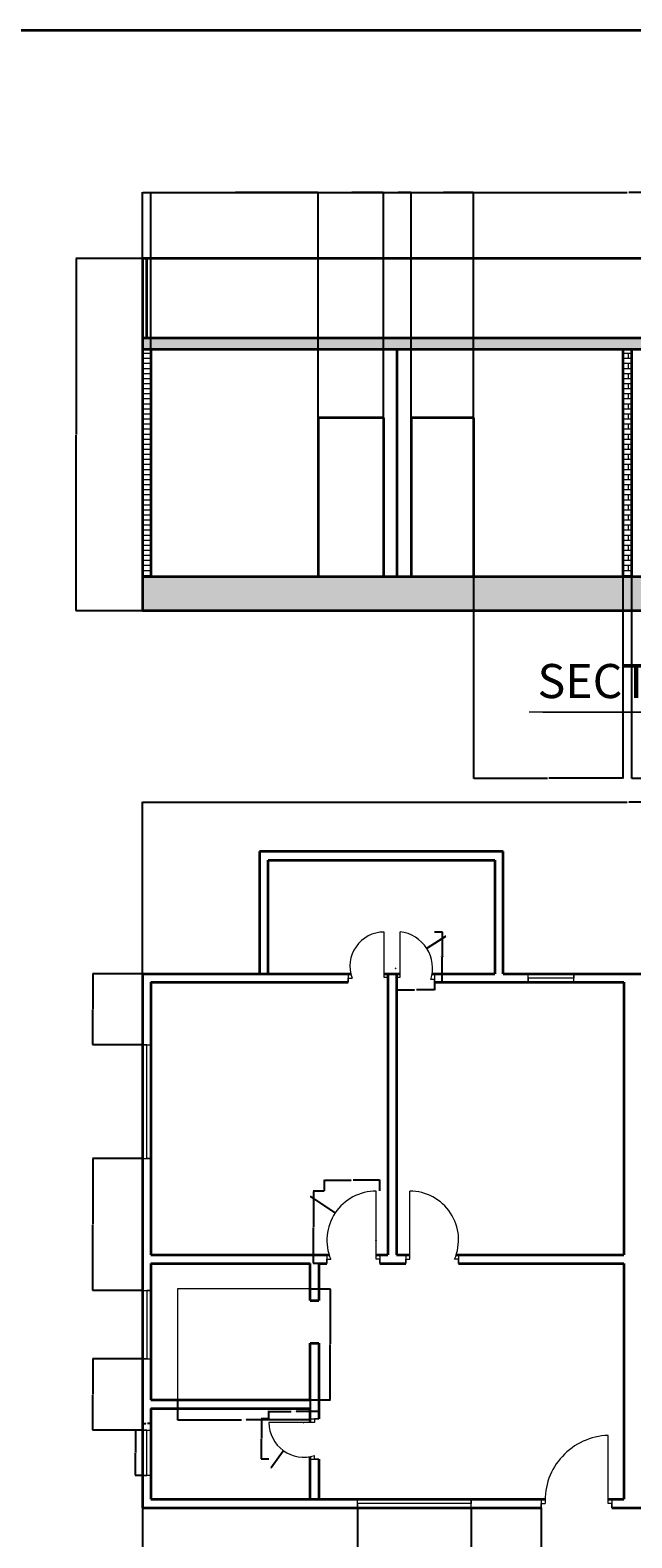
# Model space of a CAD drawing. Units: inches. Extents: x 2055 to 3558, y 1520 to 2888.
# Tile 7 of 8: x 2732 to 3050, y 2092 to 2888. Entities that reach past the tile are written whole.
import ezdxf

# ---------------------------------------------------------------- set-up
doc = ezdxf.new("R2010")
doc.units = ezdxf.units.IN
for name, color, linetype, lineweight in [('A-ANNO-DIMS', 2, 'Continuous', 18), ('A-ANNO-TEXT', 7, 'Continuous', 18), ('A-ANNO-TTLB', 7, 'Continuous', 35), ('A-DOOR', 3, 'Continuous', 18), ('A-FLOR-FIXT', 8, 'Continuous', 18), ('A-GLAZ', 4, 'Continuous', 18), ('A-SECT', 7, 'Continuous', 35), ('A-SECT-PATT', 252, 'Continuous', 13), ('A-WALL', 7, 'Continuous', 35), ('A-WALL-PATT', 252, 'Continuous', 13)]:
    doc.layers.add(name, color=color, linetype=linetype, lineweight=lineweight)
doc.styles.get("Standard").update_dxf_attribs({"font": 'arial.ttf'})
doc.dimstyles.get("Standard").update_dxf_attribs({"dimtxt": 0.18, "dimasz": 0.18, "dimexe": 0.18, "dimexo": 0.0625, "dimgap": 0.09, "dimtad": 0, "dimtih": 1, "dimtoh": 1, "dimdec": 4, "dimzin": 0, "dimdsep": 46, "dimtxsty": 'Standard', "dimcen": 0.09, "dimadec": 0, "dimazin": 0, "dimtfac": 1, "dimtdec": 4, "dimtofl": 0, "dimtmove": 0, "dimatfit": 3, "dimfxl": 1, "dimtolj": 1, "dimtzin": 0, "dimarcsym": 0})

# ---------------------------------------------------------------- blocks, each defined once
blk = doc.blocks.new('DOOR-BED-36-A')
for p, q in [((26, 2.25), (26, 38.25)), ((0, 4.5), (0, 0)), ((0, 0), (0, 2.25)), ((0, 2.25), (2, 2.25)), ((28, 2.25), (26, 2.25)), ((28, 4.5), (28, 0)), ((28, 0), (28, 2.25))]:
    blk.add_line(p, q)
blk.add_arc((26, 12.25), 26, 90, 202.62954)
blk = doc.blocks.new('DOOR-BED-36-B')
for p, q in [((2, 2.25), (2, 38.25)), ((0, 4.5), (0, 0)), ((0, 0), (0, 2.25)), ((0, 2.25), (2, 2.25)), ((27.66, 2.25), (25.66, 2.25)), ((27.66, 4.5), (27.66, 0)), ((27.66, 0), (27.66, 2.25))]:
    blk.add_line(p, q)
blk.add_arc((2, 12.47), 25.78, 336.6346, 90)
blk = doc.blocks.new('DOOR-ENTRY-36-B')
for p, q in [((35.2, 2.25), (35.2, 38.25)), ((0, 4.5), (0, 0)), ((0, 0), (0, 2.25)), ((0, 2.25), (2, 2.25)), ((37.2, 2.25), (35.2, 2.25)), ((37.2, 4.5), (37.2, 0)), ((37.2, 0), (37.2, 2.25))]:
    blk.add_line(p, q)
blk.add_arc((36.42, 3.82), 34.45, 92.03168, 182.60616)
blk = doc.blocks.new('DOOR-VERANDA-24-E')
for p, q in [((2, 2.71), (2, 26.71)), ((0, 2.71), (2, 2.71)), ((20.12, 1.44), (18.12, 1.44)), ((20.12, 4.5), (20.12, 0)), ((20.12, 0), (20.12, 1.44))]:
    blk.add_line(p, q)
blk.add_arc((-0.34, 7.44), 19.42, 342.01317, 83.06507)
blk = doc.blocks.new('DOOR-VERANDA-24-F')
for p, q in [((18.85, 2.51), (18.85, 26.51)), ((0, 4.5), (0, 0)), ((0, 0), (0, 2.25)), ((0, 2.25), (2, 2.25)), ((20.85, 2.51), (18.85, 2.51))]:
    blk.add_line(p, q)
blk.add_arc((18.85, 8.53), 17.98, 90, 200.4386)
blk = doc.blocks.new('DOOR-BATH-24-D')
for p, q in [((24, 19.33), (0, 19.33)), ((21.75, 21.33), (26.25, 21.33)), ((26.25, 21.33), (24, 21.33)), ((24, 21.33), (24, 19.33)), ((21.75, 0), (26.25, 0)), ((24, 0), (24, 2)), ((26.25, 0), (24, 0))]:
    blk.add_line(p, q)
blk.add_arc((18.26, 19.33), 18.26, 180, 288.33755)
blk = doc.blocks.new('WIN-36')
for p, q in [((2.25, 36), (0, 36)), ((0, 36), (4.5, 36)), ((2.25, 0), (2.25, 36)), ((0, 0), (4.5, 0)), ((4.5, 0), (2.25, 0))]:
    blk.add_line(p, q)
blk = doc.blocks.new('WIN-24')
for p, q in [((0, 24), (4.5, 24)), ((4.5, 24), (2.25, 24)), ((2.25, 24), (2.25, 0)), ((2.25, 0), (0, 0)), ((0, 0), (4.5, 0))]:
    blk.add_line(p, q)
blk = doc.blocks.new('WIN-24-2')
for p, q in [((2.25, 24), (0, 24)), ((0, 24), (4.5, 24)), ((2.25, 0), (2.25, 24)), ((4.5, 0), (0, 0)), ((0, 0), (2.25, 0))]:
    blk.add_line(p, q)
blk = doc.blocks.new('WIN-60')
for p, q in [((0, 60), (4.5, 60)), ((4.5, 60), (2.25, 60)), ((2.25, 60), (2.25, 0)), ((2.25, 0), (0, 0)), ((0, 0), (4.5, 0))]:
    blk.add_line(p, q)
blk = doc.blocks.new('COUNTER-1')
for p, q in [((70.02, 58.69), (0, 58.69)), ((0, 58.69), (0, 0))]:
    blk.add_line(p, q)
blk = doc.blocks.new('VERANDA-PERIMETER')
for p, q in [((0, 0), (0, 64.5)), ((4.5, 64.5), (4.5, 4.5)), ((124.15, 4.5), (124.15, 64.5)), ((128.65, 64.5), (128.65, 4.5)), ((4.5, 0), (0, 0)), ((4.5, 4.5), (124.15, 4.5)), ((128.65, 0), (4.5, 0)), ((128.65, 4.5), (128.65, 0))]:
    blk.add_line(p, q)
blk = doc.blocks.new('*D52')
at = {"layer": 'A-ANNO-DIMS', "color": 0, "lineweight": -2, "transparency": 16777216}
for p, q in [((2887.43, 2275.25), (2881.58, 2275.25)), ((2881.76, 2275.07), (2881.76, 2256.31)), ((2881.76, 2237.18), (2881.76, 2255.94)), ((2887.43, 2237), (2881.58, 2237))]:
    blk.add_line(p, q, dxfattribs=at)
at = {"layer": 'A-ANNO-DIMS', "color": 0, "transparency": 16777216}
for points in [[(2881.73, 2275.07), (2881.79, 2275.07), (2881.76, 2275.25)], [(2881.73, 2237.18), (2881.79, 2237.18), (2881.76, 2237)]]:
    blk.add_solid(points, dxfattribs=at)
at = {"layer": 'Defpoints', "color": 0, "transparency": 16777216}
for p in [(2881.76, 2275.25), (2887.49, 2275.25), (2887.49, 2237)]:
    blk.add_point(p, dxfattribs=at)
at = {"layer": 'A-ANNO-DIMS', "color": 0, "transparency": 16777216, "insert": (2881.76, 2256.12), "char_height": 0.18, "attachment_point": 5}
blk.add_mtext('\\A1;BED DOOR 38 TYP.', dxfattribs=at)
blk = doc.blocks.new('*D53')
at = {"layer": 'A-ANNO-DIMS', "color": 0, "lineweight": -2, "transparency": 16777216}
for p, q in [((2887.49, 2275.31), (2887.49, 2281.17)), ((2887.67, 2280.99), (2901.63, 2280.99)), ((2916.65, 2280.99), (2902.69, 2280.99)), ((2916.83, 2275.31), (2916.83, 2281.17))]:
    blk.add_line(p, q, dxfattribs=at)
at = {"layer": 'A-ANNO-DIMS', "color": 0, "transparency": 16777216}
for points in [[(2887.67, 2281.02), (2887.67, 2280.96), (2887.49, 2280.99)], [(2916.65, 2281.02), (2916.65, 2280.96), (2916.83, 2280.99)]]:
    blk.add_solid(points, dxfattribs=at)
at = {"layer": 'Defpoints', "color": 0, "transparency": 16777216}
for p in [(2916.83, 2280.99), (2887.49, 2275.25), (2916.83, 2275.25)]:
    blk.add_point(p, dxfattribs=at)
at = {"layer": 'A-ANNO-DIMS', "color": 0, "transparency": 16777216, "insert": (2902.16, 2280.99), "char_height": 0.18, "attachment_point": 5}
blk.add_mtext('\\A1;29 TYP.', dxfattribs=at)
blk = doc.blocks.new('*D90')
at = {"layer": 'A-ANNO-DIMS', "color": 0, "lineweight": -2, "transparency": 16777216}
for p, q in [((2945.68, 2412.21), (2949.81, 2412.21)), ((2949.63, 2412.03), (2949.63, 2399.04)), ((2949.63, 2385.68), (2949.63, 2398.67)), ((2945.68, 2385.5), (2949.81, 2385.5))]:
    blk.add_line(p, q, dxfattribs=at)
at = {"layer": 'A-ANNO-DIMS', "color": 0, "transparency": 16777216}
for points in [[(2949.6, 2412.03), (2949.66, 2412.03), (2949.63, 2412.21)], [(2949.6, 2385.68), (2949.66, 2385.68), (2949.63, 2385.5)]]:
    blk.add_solid(points, dxfattribs=at)
at = {"layer": 'Defpoints', "color": 0, "transparency": 16777216}
for p in [(2945.62, 2412.21), (2949.63, 2412.21), (2945.62, 2385.5)]:
    blk.add_point(p, dxfattribs=at)
at = {"layer": 'A-ANNO-DIMS', "color": 0, "transparency": 16777216, "insert": (2949.63, 2398.86), "char_height": 0.18, "attachment_point": 5}
blk.add_mtext('\\A1;VERANDA DOOR 27 TYP.', dxfattribs=at)
blk = doc.blocks.new('*D91')
at = {"layer": 'A-ANNO-DIMS', "color": 0, "lineweight": -2, "transparency": 16777216}
for p, q in [((2925.5, 2385.44), (2925.5, 2381.31)), ((2925.68, 2381.49), (2935.03, 2381.49)), ((2945.44, 2381.49), (2936.09, 2381.49)), ((2945.62, 2385.44), (2945.62, 2381.31))]:
    blk.add_line(p, q, dxfattribs=at)
at = {"layer": 'A-ANNO-DIMS', "color": 0, "transparency": 16777216}
for points in [[(2925.68, 2381.52), (2925.68, 2381.46), (2925.5, 2381.49)], [(2945.44, 2381.52), (2945.44, 2381.46), (2945.62, 2381.49)]]:
    blk.add_solid(points, dxfattribs=at)
at = {"layer": 'Defpoints', "color": 0, "transparency": 16777216}
for p in [(2925.5, 2385.5), (2945.62, 2385.5), (2945.62, 2381.49)]:
    blk.add_point(p, dxfattribs=at)
at = {"layer": 'A-ANNO-DIMS', "color": 0, "transparency": 16777216, "insert": (2935.56, 2381.49), "char_height": 0.18, "attachment_point": 5}
blk.add_mtext('\\A1;20 TYP.', dxfattribs=at)
blk = doc.blocks.new('*D98')
at = {"layer": 'A-ANNO-DIMS', "color": 0, "lineweight": -2, "transparency": 16777216}
for p, q in [((2858.25, 2155.07), (2858.25, 2159.12)), ((2858.43, 2158.94), (2870.06, 2158.94)), ((2884.32, 2158.94), (2872.68, 2158.94)), ((2884.5, 2155.07), (2884.5, 2159.12))]:
    blk.add_line(p, q, dxfattribs=at)
at = {"layer": 'A-ANNO-DIMS', "color": 0, "transparency": 16777216}
for points in [[(2858.43, 2158.97), (2858.43, 2158.91), (2858.25, 2158.94)], [(2884.32, 2158.97), (2884.32, 2158.91), (2884.5, 2158.94)]]:
    blk.add_solid(points, dxfattribs=at)
at = {"layer": 'Defpoints', "color": 0, "transparency": 16777216}
for p in [(2884.5, 2158.94), (2858.25, 2155), (2884.5, 2155)]:
    blk.add_point(p, dxfattribs=at)
at = {"layer": 'A-ANNO-DIMS', "color": 0, "transparency": 16777216, "insert": (2871.37, 2158.94), "char_height": 0.18, "attachment_point": 5}
blk.add_mtext('\\A1;BATH DOOR 26 TYP.', dxfattribs=at)
blk = doc.blocks.new('*D99')
at = {"layer": 'A-ANNO-DIMS', "color": 0, "lineweight": -2, "transparency": 16777216}
for p, q in [((2858.18, 2155), (2854.13, 2155)), ((2854.31, 2154.82), (2854.31, 2144.52)), ((2854.31, 2133.85), (2854.31, 2144.16)), ((2858.18, 2133.67), (2854.13, 2133.67))]:
    blk.add_line(p, q, dxfattribs=at)
at = {"layer": 'A-ANNO-DIMS', "color": 0, "transparency": 16777216}
for points in [[(2854.28, 2154.82), (2854.34, 2154.82), (2854.31, 2155)], [(2854.28, 2133.85), (2854.34, 2133.85), (2854.31, 2133.67)]]:
    blk.add_solid(points, dxfattribs=at)
at = {"layer": 'Defpoints', "color": 0, "transparency": 16777216}
for p in [(2854.31, 2155), (2858.25, 2155), (2858.25, 2133.67)]:
    blk.add_point(p, dxfattribs=at)
at = {"layer": 'A-ANNO-DIMS', "color": 0, "transparency": 16777216, "insert": (2854.31, 2144.34), "char_height": 0.18, "attachment_point": 5}
blk.add_mtext('\\A1;21 TYP.', dxfattribs=at)
blk = doc.blocks.new('*D100')
at = {"layer": 'A-ANNO-DIMS', "color": 0, "lineweight": -2, "transparency": 16777216}
for p, q in [((2791.43, 2149), (2787.72, 2149)), ((2787.9, 2148.82), (2787.9, 2137.18)), ((2787.9, 2125.18), (2787.9, 2136.82)), ((2791.43, 2125), (2787.72, 2125))]:
    blk.add_line(p, q, dxfattribs=at)
at = {"layer": 'A-ANNO-DIMS', "color": 0, "transparency": 16777216}
for points in [[(2787.87, 2148.82), (2787.93, 2148.82), (2787.9, 2149)], [(2787.87, 2125.18), (2787.93, 2125.18), (2787.9, 2125)]]:
    blk.add_solid(points, dxfattribs=at)
at = {"layer": 'Defpoints', "color": 0, "transparency": 16777216}
for p in [(2787.9, 2149), (2791.5, 2149), (2791.5, 2125)]:
    blk.add_point(p, dxfattribs=at)
at = {"layer": 'A-ANNO-DIMS', "color": 0, "transparency": 16777216, "insert": (2787.9, 2137), "char_height": 0.18, "attachment_point": 5}
blk.add_mtext('\\A1;WINDOW 24 TYP.', dxfattribs=at)
blk = doc.blocks.new('*D101')
at = {"layer": 'A-ANNO-DIMS', "color": 0, "lineweight": -2, "transparency": 16777216}
for p, q in [((2791.5, 2149.06), (2791.5, 2152.78)), ((2791.68, 2152.6), (2793.29, 2152.6)), ((2795.82, 2152.6), (2794.2, 2152.6)), ((2796, 2149.06), (2796, 2152.78))]:
    blk.add_line(p, q, dxfattribs=at)
at = {"layer": 'A-ANNO-DIMS', "color": 0, "transparency": 16777216}
for points in [[(2791.68, 2152.63), (2791.68, 2152.57), (2791.5, 2152.6)], [(2795.82, 2152.63), (2795.82, 2152.57), (2796, 2152.6)]]:
    blk.add_solid(points, dxfattribs=at)
at = {"layer": 'Defpoints', "color": 0, "transparency": 16777216}
for p in [(2796, 2152.6), (2791.5, 2149), (2796, 2149)]:
    blk.add_point(p, dxfattribs=at)
at = {"layer": 'A-ANNO-DIMS', "color": 0, "transparency": 16777216, "insert": (2793.75, 2152.6), "char_height": 0.18, "attachment_point": 5}
blk.add_mtext('\\A1;5 TYP.', dxfattribs=at)
blk = doc.blocks.new('*D106')
at = {"layer": 'A-ANNO-DIMS', "color": 0, "lineweight": -2, "transparency": 16777216}
for p, q in [((2809.98, 2164.94), (2809.98, 2154.32)), ((2880, 2164.94), (2880, 2154.32)), ((2810.16, 2154.5), (2843.8, 2154.5)), ((2879.82, 2154.5), (2846.17, 2154.5))]:
    blk.add_line(p, q, dxfattribs=at)
at = {"layer": 'A-ANNO-DIMS', "color": 0, "transparency": 16777216}
for points in [[(2810.16, 2154.53), (2810.16, 2154.47), (2809.98, 2154.5)], [(2879.82, 2154.53), (2879.82, 2154.47), (2880, 2154.5)]]:
    blk.add_solid(points, dxfattribs=at)
at = {"layer": 'Defpoints', "color": 0, "transparency": 16777216}
for p in [(2809.98, 2165), (2880, 2165), (2880, 2154.5)]:
    blk.add_point(p, dxfattribs=at)
at = {"layer": 'A-ANNO-DIMS', "color": 0, "transparency": 16777216, "insert": (2844.99, 2154.5), "char_height": 0.18, "attachment_point": 5}
blk.add_mtext('\\A1;COUNTER 70 TYP.', dxfattribs=at)
blk = doc.blocks.new('*D107')
at = {"layer": 'A-ANNO-DIMS', "color": 0, "lineweight": -2, "transparency": 16777216}
for p, q in [((2880.06, 2223.69), (2890.68, 2223.69)), ((2890.5, 2223.51), (2890.5, 2194.53)), ((2890.5, 2165.18), (2890.5, 2194.16)), ((2880.06, 2165), (2890.68, 2165))]:
    blk.add_line(p, q, dxfattribs=at)
at = {"layer": 'A-ANNO-DIMS', "color": 0, "transparency": 16777216}
for points in [[(2890.47, 2223.51), (2890.53, 2223.51), (2890.5, 2223.69)], [(2890.47, 2165.18), (2890.53, 2165.18), (2890.5, 2165)]]:
    blk.add_solid(points, dxfattribs=at)
at = {"layer": 'Defpoints', "color": 0, "transparency": 16777216}
for p in [(2880, 2223.69), (2890.5, 2223.69), (2880, 2165)]:
    blk.add_point(p, dxfattribs=at)
at = {"layer": 'A-ANNO-DIMS', "color": 0, "transparency": 16777216, "insert": (2890.5, 2194.34), "char_height": 0.18, "attachment_point": 5}
blk.add_mtext('\\A1;59 TYP.', dxfattribs=at)
blk = doc.blocks.new('*D124')
at = {"layer": 'A-ANNO-DIMS', "color": 0, "lineweight": -2, "transparency": 16777216}
for p, q in [((2791.5, 2390.06), (2791.5, 2480.78)), ((2791.68, 2480.6), (3047.35, 2480.6)), ((3303.82, 2480.6), (3048.14, 2480.6)), ((3304, 2390.06), (3304, 2480.78))]:
    blk.add_line(p, q, dxfattribs=at)
at = {"layer": 'A-ANNO-DIMS', "color": 0, "transparency": 16777216}
for points in [[(2791.68, 2480.63), (2791.68, 2480.57), (2791.5, 2480.6)], [(3303.82, 2480.63), (3303.82, 2480.57), (3304, 2480.6)]]:
    blk.add_solid(points, dxfattribs=at)
at = {"layer": 'Defpoints', "color": 0, "transparency": 16777216}
for p in [(3304, 2480.6), (2791.5, 2390), (3304, 2390)]:
    blk.add_point(p, dxfattribs=at)
at = {"layer": 'A-ANNO-DIMS', "color": 0, "transparency": 16777216, "insert": (3047.75, 2480.6), "char_height": 0.18, "attachment_point": 5}
blk.add_mtext('\\A1;512.5', dxfattribs=at)
blk = doc.blocks.new('*D128')
at = {"layer": 'A-ANNO-DIMS', "color": 0, "lineweight": -2, "transparency": 16777216}
for p, q in [((2791.5, 2107.94), (2791.5, 2081.72)), ((2904.9, 2107.94), (2904.9, 2081.72)), ((2791.68, 2081.9), (2847.81, 2081.9)), ((2904.72, 2081.9), (2848.58, 2081.9))]:
    blk.add_line(p, q, dxfattribs=at)
at = {"layer": 'A-ANNO-DIMS', "color": 0, "transparency": 16777216}
for points in [[(2791.68, 2081.93), (2791.68, 2081.87), (2791.5, 2081.9)], [(2904.72, 2081.93), (2904.72, 2081.87), (2904.9, 2081.9)]]:
    blk.add_solid(points, dxfattribs=at)
at = {"layer": 'Defpoints', "color": 0, "transparency": 16777216}
for p in [(2791.5, 2108), (2904.9, 2108), (2904.9, 2081.9)]:
    blk.add_point(p, dxfattribs=at)
at = {"layer": 'A-ANNO-DIMS', "color": 0, "transparency": 16777216, "insert": (2848.2, 2081.9), "char_height": 0.18, "attachment_point": 5}
blk.add_mtext('\\A1;113.4', dxfattribs=at)
blk = doc.blocks.new('*D129')
at = {"layer": 'A-ANNO-DIMS', "color": 0, "lineweight": -2, "transparency": 16777216}
for p, q in [((2964.9, 2107.94), (2964.9, 2081.72)), ((3001.98, 2107.94), (3001.98, 2081.72)), ((2965.08, 2081.9), (2983.05, 2081.9)), ((3001.8, 2081.9), (2983.83, 2081.9))]:
    blk.add_line(p, q, dxfattribs=at)
at = {"layer": 'A-ANNO-DIMS', "color": 0, "transparency": 16777216}
for points in [[(2965.08, 2081.93), (2965.08, 2081.87), (2964.9, 2081.9)], [(3001.8, 2081.93), (3001.8, 2081.87), (3001.98, 2081.9)]]:
    blk.add_solid(points, dxfattribs=at)
at = {"layer": 'Defpoints', "color": 0, "transparency": 16777216}
for p in [(2964.9, 2108), (3001.98, 2108), (3001.98, 2081.9)]:
    blk.add_point(p, dxfattribs=at)
at = {"layer": 'A-ANNO-DIMS', "color": 0, "transparency": 16777216, "insert": (2983.44, 2081.9), "char_height": 0.18, "attachment_point": 5}
blk.add_mtext('\\A1;37.08', dxfattribs=at)
blk = doc.blocks.new('*D130')
at = {"layer": 'A-ANNO-DIMS', "color": 0, "lineweight": -2, "transparency": 16777216}
for p, q in [((2791.43, 2186.72), (2765.22, 2186.72)), ((2765.4, 2186.54), (2765.4, 2168.04)), ((2765.4, 2149.18), (2765.4, 2167.68)), ((2791.43, 2149), (2765.22, 2149))]:
    blk.add_line(p, q, dxfattribs=at)
at = {"layer": 'A-ANNO-DIMS', "color": 0, "transparency": 16777216}
for points in [[(2765.37, 2186.54), (2765.43, 2186.54), (2765.4, 2186.72)], [(2765.37, 2149.18), (2765.43, 2149.18), (2765.4, 2149)]]:
    blk.add_solid(points, dxfattribs=at)
at = {"layer": 'Defpoints', "color": 0, "transparency": 16777216}
for p in [(2765.4, 2186.72), (2791.5, 2186.72), (2791.5, 2149)]:
    blk.add_point(p, dxfattribs=at)
at = {"layer": 'A-ANNO-DIMS', "color": 0, "transparency": 16777216, "insert": (2765.4, 2167.86), "char_height": 0.18, "attachment_point": 5}
blk.add_mtext('\\A1;37.72', dxfattribs=at)
blk = doc.blocks.new('*D131')
at = {"layer": 'A-ANNO-DIMS', "color": 0, "lineweight": -2, "transparency": 16777216}
for p, q in [((2791.43, 2292.52), (2765.22, 2292.52)), ((2765.4, 2292.34), (2765.4, 2257.8)), ((2765.4, 2222.9), (2765.4, 2257.44)), ((2791.43, 2222.72), (2765.22, 2222.72))]:
    blk.add_line(p, q, dxfattribs=at)
at = {"layer": 'A-ANNO-DIMS', "color": 0, "transparency": 16777216}
for points in [[(2765.37, 2292.34), (2765.43, 2292.34), (2765.4, 2292.52)], [(2765.37, 2222.9), (2765.43, 2222.9), (2765.4, 2222.72)]]:
    blk.add_solid(points, dxfattribs=at)
at = {"layer": 'Defpoints', "color": 0, "transparency": 16777216}
for p in [(2765.4, 2292.52), (2791.5, 2292.52), (2791.5, 2222.72)]:
    blk.add_point(p, dxfattribs=at)
at = {"layer": 'A-ANNO-DIMS', "color": 0, "transparency": 16777216, "insert": (2765.4, 2257.62), "char_height": 0.18, "attachment_point": 5}
blk.add_mtext('\\A1;69.8', dxfattribs=at)
blk = doc.blocks.new('*D132')
at = {"layer": 'A-ANNO-DIMS', "color": 0, "lineweight": -2, "transparency": 16777216}
for p, q in [((2791.43, 2390), (2765.22, 2390)), ((2765.4, 2389.82), (2765.4, 2371.44)), ((2765.4, 2352.7), (2765.4, 2371.08)), ((2791.43, 2352.52), (2765.22, 2352.52))]:
    blk.add_line(p, q, dxfattribs=at)
at = {"layer": 'A-ANNO-DIMS', "color": 0, "transparency": 16777216}
for points in [[(2765.37, 2389.82), (2765.43, 2389.82), (2765.4, 2390)], [(2765.37, 2352.7), (2765.43, 2352.7), (2765.4, 2352.52)]]:
    blk.add_solid(points, dxfattribs=at)
at = {"layer": 'Defpoints', "color": 0, "transparency": 16777216}
for p in [(2765.4, 2390), (2791.5, 2390), (2791.5, 2352.52)]:
    blk.add_point(p, dxfattribs=at)
at = {"layer": 'A-ANNO-DIMS', "color": 0, "transparency": 16777216, "insert": (2765.4, 2371.26), "char_height": 0.18, "attachment_point": 5}
blk.add_mtext('\\A1;37.48', dxfattribs=at)
blk = doc.blocks.new('*D149')
at = {"layer": 'A-ANNO-DIMS', "color": 0, "lineweight": -2, "transparency": 16777216}
for p, q in [((2791.5, 2767.66), (2791.5, 2802.68)), ((2791.68, 2802.5), (3047.35, 2802.5)), ((3303.82, 2802.5), (3048.14, 2802.5)), ((3304, 2767.66), (3304, 2802.68))]:
    blk.add_line(p, q, dxfattribs=at)
at = {"layer": 'A-ANNO-DIMS', "color": 0, "transparency": 16777216}
for points in [[(2791.68, 2802.53), (2791.68, 2802.47), (2791.5, 2802.5)], [(3303.82, 2802.53), (3303.82, 2802.47), (3304, 2802.5)]]:
    blk.add_solid(points, dxfattribs=at)
at = {"layer": 'Defpoints', "color": 0, "transparency": 16777216}
for p in [(3304, 2802.5), (2791.5, 2767.6), (3304, 2767.6)]:
    blk.add_point(p, dxfattribs=at)
at = {"layer": 'A-ANNO-DIMS', "color": 0, "transparency": 16777216, "insert": (3047.75, 2802.5), "char_height": 0.18, "attachment_point": 5}
blk.add_mtext('\\A1;512.5', dxfattribs=at)
blk = doc.blocks.new('*D150')
at = {"layer": 'A-ANNO-DIMS', "color": 0, "lineweight": -2, "transparency": 16777216}
for p, q in [((2791.43, 2767.6), (2756.42, 2767.6)), ((2756.6, 2767.42), (2756.6, 2674.78)), ((2756.6, 2581.78), (2756.6, 2674.42)), ((2791.43, 2581.6), (2756.42, 2581.6))]:
    blk.add_line(p, q, dxfattribs=at)
at = {"layer": 'A-ANNO-DIMS', "color": 0, "transparency": 16777216}
for points in [[(2756.57, 2767.42), (2756.63, 2767.42), (2756.6, 2767.6)], [(2756.57, 2581.78), (2756.63, 2581.78), (2756.6, 2581.6)]]:
    blk.add_solid(points, dxfattribs=at)
at = {"layer": 'Defpoints', "color": 0, "transparency": 16777216}
for p in [(2756.6, 2767.6), (2791.5, 2767.6), (2791.5, 2581.6)]:
    blk.add_point(p, dxfattribs=at)
at = {"layer": 'A-ANNO-DIMS', "color": 0, "transparency": 16777216, "insert": (2756.6, 2674.6), "char_height": 0.18, "attachment_point": 5}
blk.add_mtext('\\A1;186', dxfattribs=at)
blk = doc.blocks.new('*D151')
at = {"layer": 'A-ANNO-DIMS', "color": 0, "lineweight": -2, "transparency": 16777216}
for p, q in [((2796, 2599.66), (2796, 2802.68)), ((2796.18, 2802.5), (2839.76, 2802.5)), ((2884.13, 2802.5), (2840.55, 2802.5)), ((2884.31, 2599.66), (2884.31, 2802.68))]:
    blk.add_line(p, q, dxfattribs=at)
at = {"layer": 'A-ANNO-DIMS', "color": 0, "transparency": 16777216}
for points in [[(2796.18, 2802.53), (2796.18, 2802.47), (2796, 2802.5)], [(2884.13, 2802.53), (2884.13, 2802.47), (2884.31, 2802.5)]]:
    blk.add_solid(points, dxfattribs=at)
at = {"layer": 'Defpoints', "color": 0, "transparency": 16777216}
for p in [(2884.31, 2802.5), (2796, 2599.6), (2884.31, 2599.6)]:
    blk.add_point(p, dxfattribs=at)
at = {"layer": 'A-ANNO-DIMS', "color": 0, "transparency": 16777216, "insert": (2840.15, 2802.5), "char_height": 0.18, "attachment_point": 5}
blk.add_mtext('\\A1;88.32', dxfattribs=at)
blk = doc.blocks.new('*D152')
at = {"layer": 'A-ANNO-DIMS', "color": 0, "lineweight": -2, "transparency": 16777216}
for p, q in [((3045, 2719.54), (3045, 2493.05)), ((2966.24, 2683.54), (2966.24, 2493.05)), ((2966.42, 2493.23), (3005.23, 2493.23)), ((3044.82, 2493.23), (3006.01, 2493.23))]:
    blk.add_line(p, q, dxfattribs=at)
at = {"layer": 'A-ANNO-DIMS', "color": 0, "transparency": 16777216}
for points in [[(2966.42, 2493.26), (2966.42, 2493.2), (2966.24, 2493.23)], [(3044.82, 2493.26), (3044.82, 2493.2), (3045, 2493.23)]]:
    blk.add_solid(points, dxfattribs=at)
at = {"layer": 'Defpoints', "color": 0, "transparency": 16777216}
for p in [(3045, 2719.6), (2966.24, 2683.6), (3045, 2493.23)]:
    blk.add_point(p, dxfattribs=at)
at = {"layer": 'A-ANNO-DIMS', "color": 0, "transparency": 16777216, "insert": (3005.62, 2493.23), "char_height": 0.18, "attachment_point": 5}
blk.add_mtext('\\A1;78.75', dxfattribs=at)
blk = doc.blocks.new('*D153')
at = {"layer": 'A-ANNO-DIMS', "color": 0, "lineweight": -2, "transparency": 16777216}
for p, q in [((3049.5, 2719.54), (3049.5, 2493.05)), ((3116.25, 2683.54), (3116.25, 2493.05)), ((3049.68, 2493.23), (3082.48, 2493.23)), ((3116.07, 2493.23), (3083.27, 2493.23))]:
    blk.add_line(p, q, dxfattribs=at)
at = {"layer": 'A-ANNO-DIMS', "color": 0, "transparency": 16777216}
for points in [[(3049.68, 2493.26), (3049.68, 2493.2), (3049.5, 2493.23)], [(3116.07, 2493.26), (3116.07, 2493.2), (3116.25, 2493.23)]]:
    blk.add_solid(points, dxfattribs=at)
at = {"layer": 'Defpoints', "color": 0, "transparency": 16777216}
for p in [(3049.5, 2719.6), (3116.25, 2683.6), (3116.25, 2493.23)]:
    blk.add_point(p, dxfattribs=at)
at = {"layer": 'A-ANNO-DIMS', "color": 0, "transparency": 16777216, "insert": (3082.87, 2493.23), "char_height": 0.18, "attachment_point": 5}
blk.add_mtext('\\A1;66.76', dxfattribs=at)
blk = doc.blocks.new('*D154')
at = {"layer": 'A-ANNO-DIMS', "color": 0, "lineweight": -2, "transparency": 16777216}
for p, q in [((2884.31, 2683.66), (2884.31, 2802.68)), ((2884.49, 2802.5), (2901.05, 2802.5)), ((2918.55, 2802.5), (2901.98, 2802.5)), ((2918.73, 2683.66), (2918.73, 2802.68))]:
    blk.add_line(p, q, dxfattribs=at)
at = {"layer": 'A-ANNO-DIMS', "color": 0, "transparency": 16777216}
for points in [[(2884.49, 2802.53), (2884.49, 2802.47), (2884.31, 2802.5)], [(2918.55, 2802.53), (2918.55, 2802.47), (2918.73, 2802.5)]]:
    blk.add_solid(points, dxfattribs=at)
at = {"layer": 'Defpoints', "color": 0, "transparency": 16777216}
for p in [(2918.73, 2802.5), (2884.31, 2683.6), (2918.73, 2683.6)]:
    blk.add_point(p, dxfattribs=at)
at = {"layer": 'A-ANNO-DIMS', "color": 0, "transparency": 16777216, "insert": (2901.52, 2802.5), "char_height": 0.18, "attachment_point": 5}
blk.add_mtext('\\A1;34.415', dxfattribs=at)
blk = doc.blocks.new('*D155')
at = {"layer": 'A-ANNO-DIMS', "color": 0, "lineweight": -2, "transparency": 16777216}
for p, q in [((2918.73, 2683.66), (2918.73, 2802.68)), ((2918.91, 2802.5), (2925.6, 2802.5)), ((2933.21, 2802.5), (2926.51, 2802.5)), ((2933.39, 2683.66), (2933.39, 2802.68))]:
    blk.add_line(p, q, dxfattribs=at)
at = {"layer": 'A-ANNO-DIMS', "color": 0, "transparency": 16777216}
for points in [[(2918.91, 2802.53), (2918.91, 2802.47), (2918.73, 2802.5)], [(2933.21, 2802.53), (2933.21, 2802.47), (2933.39, 2802.5)]]:
    blk.add_solid(points, dxfattribs=at)
at = {"layer": 'Defpoints', "color": 0, "transparency": 16777216}
for p in [(2933.39, 2802.5), (2918.73, 2683.6), (2933.39, 2683.6)]:
    blk.add_point(p, dxfattribs=at)
at = {"layer": 'A-ANNO-DIMS', "color": 0, "transparency": 16777216, "insert": (2926.06, 2802.5), "char_height": 0.18, "attachment_point": 5}
blk.add_mtext('\\A1;14.663', dxfattribs=at)
blk = doc.blocks.new('*D156')
at = {"layer": 'A-ANNO-DIMS', "color": 0, "lineweight": -2, "transparency": 16777216}
for p, q in [((2933.39, 2683.66), (2933.39, 2802.68)), ((2933.57, 2802.5), (2949.35, 2802.5)), ((2966.06, 2802.5), (2950.28, 2802.5)), ((2966.24, 2683.66), (2966.24, 2802.68))]:
    blk.add_line(p, q, dxfattribs=at)
at = {"layer": 'A-ANNO-DIMS', "color": 0, "transparency": 16777216}
for points in [[(2933.57, 2802.53), (2933.57, 2802.47), (2933.39, 2802.5)], [(2966.06, 2802.53), (2966.06, 2802.47), (2966.24, 2802.5)]]:
    blk.add_solid(points, dxfattribs=at)
at = {"layer": 'Defpoints', "color": 0, "transparency": 16777216}
for p in [(2966.24, 2802.5), (2933.39, 2683.6), (2966.24, 2683.6)]:
    blk.add_point(p, dxfattribs=at)
at = {"layer": 'A-ANNO-DIMS', "color": 0, "transparency": 16777216, "insert": (2949.82, 2802.5), "char_height": 0.18, "attachment_point": 5}
blk.add_mtext('\\A1;32.856', dxfattribs=at)
blk = doc.blocks.new('*D164')
at = {"layer": 'A-ANNO-DIMS', "color": 0, "lineweight": -2, "transparency": 16777216}
for p, q in [((2880.04, 2272.32), (2880.22, 2272.32)), ((2880.22, 2272.32), (2893.05, 2263.77)), ((2914.74, 2249.25), (2914.92, 2249.25)), ((2914.83, 2249.16), (2914.83, 2249.34))]:
    blk.add_line(p, q, dxfattribs=at)
at = {"layer": 'A-ANNO-DIMS', "color": 0, "transparency": 16777216}
blk.add_solid([(2893.07, 2263.8), (2893.04, 2263.75), (2893.2, 2263.67)], dxfattribs=at)
at = {"layer": 'Defpoints', "color": 0, "transparency": 16777216}
for p in [(2893.2, 2263.67), (2914.83, 2249.25)]:
    blk.add_point(p, dxfattribs=at)
at = {"layer": 'A-ANNO-DIMS', "color": 0, "transparency": 16777216, "insert": (2879.49, 2272.32), "char_height": 0.18, "attachment_point": 5}
blk.add_mtext('\\A1;R25.997', dxfattribs=at)
blk = doc.blocks.new('*D170')
at = {"layer": 'A-ANNO-DIMS', "color": 0, "lineweight": -2, "transparency": 16777216}
for p, q in [((2951.34, 2409.65), (2941.67, 2403.48)), ((2951.52, 2409.65), (2951.34, 2409.65)), ((2925.06, 2392.94), (2925.24, 2392.94)), ((2925.15, 2392.85), (2925.15, 2393.03))]:
    blk.add_line(p, q, dxfattribs=at)
at = {"layer": 'A-ANNO-DIMS', "color": 0, "transparency": 16777216}
blk.add_solid([(2941.66, 2403.5), (2941.69, 2403.45), (2941.52, 2403.38)], dxfattribs=at)
at = {"layer": 'Defpoints', "color": 0, "transparency": 16777216}
for p in [(2941.52, 2403.38), (2925.15, 2392.94)]:
    blk.add_point(p, dxfattribs=at)
at = {"layer": 'A-ANNO-DIMS', "color": 0, "transparency": 16777216, "insert": (2952.07, 2409.65), "char_height": 0.18, "attachment_point": 5}
blk.add_mtext('\\A1;R19.417', dxfattribs=at)
blk = doc.blocks.new('*D171')
at = {"layer": 'A-ANNO-DIMS', "color": 0, "lineweight": -2, "transparency": 16777216}
for p, q in [((2876.41, 2153), (2876.59, 2153)), ((2876.5, 2152.91), (2876.5, 2153.09)), ((2859.4, 2129.32), (2865.71, 2138.06)), ((2859.22, 2129.32), (2859.4, 2129.32))]:
    blk.add_line(p, q, dxfattribs=at)
at = {"layer": 'A-ANNO-DIMS', "color": 0, "transparency": 16777216}
blk.add_solid([(2865.69, 2138.07), (2865.73, 2138.04), (2865.81, 2138.2)], dxfattribs=at)
at = {"layer": 'Defpoints', "color": 0, "transparency": 16777216}
for p in [(2876.5, 2153), (2865.81, 2138.2)]:
    blk.add_point(p, dxfattribs=at)
at = {"layer": 'A-ANNO-DIMS', "color": 0, "transparency": 16777216, "insert": (2858.67, 2129.32), "char_height": 0.18, "attachment_point": 5}
blk.add_mtext('\\A1;R18.256', dxfattribs=at)

msp = doc.modelspace()

# ---------------------------------------------------------------- hatches: boundary and pattern name
at = {"layer": 'A-SECT-PATT'}
h = msp.add_hatch(dxfattribs=at)
h.set_pattern_fill('AR-CONC', color=256, scale=0.0531496, style=0)
h.paths.add_polyline_path([(2791.4955, 2719.5987), (3303.9955, 2719.5987), (3303.9955, 2725.5987), (2791.4955, 2725.5987)])
h = msp.add_hatch(dxfattribs=at)
h.set_pattern_fill('AR-CONC', color=256, scale=0.07874016, style=0)
h.paths.add_polyline_path([(2791.4955, 2581.5987), (3303.9955, 2581.5987), (3303.9955, 2599.5987), (2791.4955, 2599.5987)])
at = {"layer": 'A-WALL-PATT'}
h = msp.add_hatch(dxfattribs=at)
h.set_pattern_fill('AR-BRSTD', color=256, scale=0.03937008, style=0)
h.paths.add_polyline_path([(2791.4955, 2599.5987), (2795.9955, 2599.5987), (2795.9955, 2719.5987), (2791.4955, 2719.5987)])
h = msp.add_hatch(dxfattribs=at)
h.set_pattern_fill('AR-BRSTD', color=256, scale=0.03937008, style=0)
h.paths.add_polyline_path([(3044.9955, 2599.5987), (3049.4955, 2599.5987), (3049.4955, 2719.5987), (3044.9955, 2719.5987)])

# ---------------------------------------------------------------- linework, layer by layer
at = {"layer": 'A-ANNO-TEXT'}
for p, q in [((3138.6573, 2528.1346), (2995.5972, 2528.1346)), ((3002.7098, 2528.1346), (3138.6573, 2528.1346))]:
    msp.add_line(p, q, dxfattribs=at)
at = {"layer": 'A-ANNO-TTLB'}
msp.add_lwpolyline([(2054.7598, 2888.2545), (3557.8479, 2888.2545), (3557.8479, 1520.3256), (2054.7598, 1520.3256)], close=True, dxfattribs=at)
at = {"layer": 'A-SECT'}
for p, q in [((2791.4955, 2767.5987), (2791.4955, 2581.5987)), ((3303.9955, 2767.5987), (2791.4955, 2767.5987)), ((2793.7455, 2725.5987), (2793.7455, 2767.5987)), ((3303.9955, 2725.5987), (2791.4955, 2725.5987)), ((3303.9955, 2719.5987), (2791.4955, 2719.5987)), ((2795.9955, 2719.5987), (2795.9955, 2599.5987)), ((2925.831, 2599.5987), (2925.831, 2719.5987)), ((3044.9955, 2719.5987), (3044.9955, 2599.5987)), ((3049.4955, 2719.5987), (3049.4955, 2599.5987)), ((2884.3106, 2683.5987), (2884.3106, 2599.5987)), ((2918.7261, 2683.5987), (2884.3106, 2683.5987)), ((2918.7261, 2683.5987), (2918.7261, 2599.5987)), ((2933.3886, 2683.5987), (2933.3886, 2599.5987)), ((2966.2445, 2683.5987), (2933.3886, 2683.5987)), ((2966.2445, 2683.5987), (2966.2445, 2599.5987)), ((3303.9955, 2599.5987), (2791.4955, 2599.5987)), ((3303.9955, 2581.5987), (2791.4955, 2581.5987))]:
    msp.add_line(p, q, dxfattribs=at)
at = {"layer": 'A-WALL'}
for p, q in [((2791.4955, 2389.9995), (2901.4693, 2389.9995)), ((2791.4955, 2389.9995), (2853.2676, 2389.9995)), ((2791.4955, 2389.9995), (2791.4955, 2107.9995)), ((2857.7676, 2389.9995), (2901.4693, 2389.9995)), ((2918.9955, 2389.9995), (2927.4955, 2389.9995)), ((2918.9955, 2389.9995), (2927.4955, 2389.9995)), ((2920.9955, 2389.9995), (2920.9955, 2241.4995)), ((2925.4955, 2389.9995), (2925.4955, 2241.4995)), ((2944.3448, 2389.9995), (2977.4137, 2389.9995)), ((2944.3448, 2389.9995), (2977.4137, 2389.9995)), ((2981.9137, 2389.9995), (3111.0777, 2389.9995)), ((2981.9137, 2389.9995), (3111.0777, 2389.9995)), ((2795.9955, 2385.4995), (2900.1441, 2385.4995)), ((2795.9955, 2385.4995), (2795.9955, 2241.4995)), ((2945.6194, 2385.4995), (3045.4955, 2385.4995)), ((3045.4955, 2385.4995), (3045.4955, 2241.4995)), ((2795.9955, 2241.4995), (2890.0198, 2241.4995)), ((2879.9955, 2241.4995), (2884.4955, 2241.4995)), ((2914.8339, 2241.4995), (2920.9955, 2241.4995)), ((2925.4955, 2241.4995), (2932.5344, 2241.4995)), ((2957.0474, 2241.4995), (3045.4955, 2241.4995)), ((2795.9955, 2236.9995), (2879.9955, 2236.9995)), ((2795.9955, 2236.9995), (2795.9955, 2164.9995)), ((2879.9955, 2217.4337), (2879.9955, 2236.9995)), ((2884.4955, 2236.9995), (2888.8383, 2236.9995)), ((2884.4955, 2236.9995), (2884.4955, 2217.4337)), ((2916.8339, 2236.9995), (2930.5344, 2236.9995)), ((2958.1976, 2236.9995), (3045.4955, 2236.9995)), ((3045.4955, 2236.9995), (3045.4955, 2112.4995)), ((2879.9955, 2217.4337), (2884.4955, 2217.4337)), ((2879.9955, 2164.9995), (2879.9955, 2194.987)), ((2879.9955, 2194.987), (2884.4955, 2194.987)), ((2884.4955, 2194.987), (2884.4955, 2155.0034)), ((2795.9955, 2164.9995), (2879.9955, 2164.9995)), ((2795.9955, 2160.4995), (2879.9955, 2160.4995)), ((2795.9955, 2160.4995), (2795.9955, 2112.4995)), ((2879.9955, 2153.0034), (2879.9955, 2160.4995)), ((2879.9955, 2112.4995), (2879.9955, 2135.0845)), ((2884.4955, 2133.6742), (2884.4955, 2112.4995)), ((2795.9955, 2112.4995), (3003.9524, 2112.4995)), ((2795.9955, 2112.4995), (2879.9955, 2112.4995)), ((3037.1791, 2112.4995), (3045.4955, 2112.4995)), ((2791.4955, 2107.9995), (3001.9813, 2107.9995)), ((2791.4955, 2107.9995), (3001.9813, 2107.9995)), ((3039.1791, 2107.9995), (3045.4955, 2107.9995)), ((3039.1791, 2107.9995), (3055.5099, 2107.9995))]:
    msp.add_line(p, q, dxfattribs=at)

# ---------------------------------------------------------------- block references
at = {"layer": 'A-DOOR'}
for name, p in [('DOOR-VERANDA-24-F', (2900.1438, 2385.499)), ('DOOR-VERANDA-24-E', (2925.4958, 2385.499)), ('DOOR-BED-36-A', (2888.8368, 2236.999)), ('DOOR-BED-36-B', (2930.5348, 2236.999)), ('DOOR-BATH-24-D', (2858.2458, 2133.674)), ('DOOR-ENTRY-36-B', (3001.9808, 2107.999))]:
    msp.add_blockref(name, p, dxfattribs=at)
at = {"layer": 'A-FLOR-FIXT'}
msp.add_blockref('COUNTER-1', (2809.9768, 2164.999), dxfattribs=at)
at = {"layer": 'A-GLAZ', "extrusion": (0, 0, -1), "zscale": -1}
for name, p, rotation in [('WIN-24', (-2995.0866, 2385.4998), 90), ('WIN-60', (-2791.4958, 2352.516), 180), ('WIN-36', (-2791.4958, 2222.7217), 180), ('WIN-60', (-2904.9008, 2107.9998), 90)]:
    msp.add_blockref(name, p, dxfattribs=dict(at, rotation=rotation))
at = {"layer": 'A-GLAZ'}
msp.add_blockref('WIN-24-2', (2791.4958, 2124.998), dxfattribs=at)
at = {"layer": 'A-WALL', "extrusion": (0, 0, -1), "zscale": -1, "rotation": 180}
msp.add_blockref('VERANDA-PERIMETER', (-2853.2676, 2454.5), dxfattribs=at)

# ---------------------------------------------------------------- texts
at = {"layer": 'A-ANNO-TEXT', "insert": (2999.9928, 2553.5585), "char_height": 18, "attachment_point": 1}
msp.add_mtext_dynamic_manual_height_columns('SECTION-A', width=543.632331, gutter_width=12.5, heights=[0], dxfattribs=at)

# ---------------------------------------------------------------- dimensions: what is measured, and where the dimension line sits
at = {"layer": 'A-ANNO-DIMS'}
for base, p1, p2, override, picture, middle in [((3303.9955, 2802.4987), (2791.4955, 2767.5987), (3303.9955, 2767.5987), {"dimdec": 1, "dimlfac": 1, "dimrnd": 0, "dimzin": 0, "dimdsep": 46, "dimlunit": 2}, '*D149', (3047.7455, 2802.4987)), ((2884.3106, 2802.4987), (2795.9955, 2599.5987), (2884.3106, 2599.5987), {"dimdec": 2, "dimlfac": 1, "dimrnd": 0, "dimzin": 0, "dimdsep": 46, "dimlunit": 2}, '*D151', (2840.1531, 2802.4987)), ((2918.72609, 2802.49869), (2884.31064, 2683.59869), (2918.72609, 2683.59869), {"dimdec": 3, "dimlfac": 1, "dimrnd": 0, "dimzin": 0, "dimdsep": 46, "dimlunit": 2}, '*D154', (2901.51836, 2802.49869)), ((2933.3886, 2802.49869), (2918.72609, 2683.59869), (2933.3886, 2683.59869), {"dimdec": 3, "dimlfac": 1, "dimrnd": 0, "dimzin": 0, "dimdsep": 46, "dimlunit": 2}, '*D155', (2926.05735, 2802.49869)), ((2966.2445, 2802.4987), (2933.3886, 2683.5987), (2966.2445, 2683.5987), {"dimdec": 3, "dimlfac": 1, "dimrnd": 0, "dimzin": 0, "dimdsep": 46, "dimlunit": 2}, '*D156', (2949.8165, 2802.4987)), ((3044.9955, 2493.2346), (2966.2445, 2683.5987), (3044.9955, 2719.5987), {"dimdec": 2, "dimlfac": 1, "dimrnd": 0, "dimzin": 0, "dimdsep": 46, "dimlunit": 2}, '*D152', (3005.62, 2493.2346)), ((3116.2543, 2493.2346), (3049.4955, 2719.5987), (3116.2543, 2683.5987), {"dimdec": 2, "dimlfac": 1, "dimrnd": 0, "dimzin": 0, "dimdsep": 46, "dimlunit": 2}, '*D153', (3082.8749, 2493.2346)), ((3303.9955, 2480.5995), (2791.4955, 2389.9995), (3303.9955, 2389.9995), {"dimdec": 1, "dimlfac": 1, "dimrnd": 0, "dimzin": 0, "dimdsep": 46, "dimlunit": 2}, '*D124', (3047.7455, 2480.5995)), ((2904.9009, 2081.8995), (2791.4955, 2107.9995), (2904.9009, 2107.9995), {"dimdec": 1, "dimlfac": 1, "dimrnd": 0, "dimzin": 0, "dimdsep": 46, "dimlunit": 2}, '*D128', (2848.1982, 2081.8995)), ((3001.9813, 2081.8995), (2964.9009, 2107.9995), (3001.9813, 2107.9995), {"dimdec": 2, "dimlfac": 1, "dimrnd": 0, "dimzin": 0, "dimdsep": 46, "dimlunit": 2}, '*D129', (2983.4411, 2081.8995))]:
    dim = msp.add_linear_dim(base=base, p1=p1, p2=p2, dimstyle='Standard', override=override, dxfattribs=at)
    dim.commit()
    dim.dimension.update_dxf_attribs({"geometry": picture, "text_midpoint": middle})
for base, p1, p2, override, picture, middle in [((2756.5955, 2767.5987), (2791.4955, 2581.5987), (2791.4955, 2767.5987), {"dimdec": 0, "dimlfac": 1, "dimrnd": 0, "dimzin": 0, "dimdsep": 46, "dimlunit": 2}, '*D150', (2756.5955, 2674.5987)), ((2765.3955, 2389.9995), (2791.4955, 2352.5159), (2791.4955, 2389.9995), {"dimdec": 2, "dimlfac": 1, "dimrnd": 0, "dimzin": 0, "dimdsep": 46, "dimlunit": 2}, '*D132', (2765.3955, 2371.2577)), ((2765.3955, 2292.5159), (2791.4955, 2222.7216), (2791.4955, 2292.5159), {"dimdec": 1, "dimlfac": 1, "dimrnd": 0, "dimzin": 0, "dimdsep": 46, "dimlunit": 2}, '*D131', (2765.3955, 2257.6187)), ((2765.3955, 2186.7216), (2791.4955, 2148.9982), (2791.4955, 2186.7216), {"dimdec": 2, "dimlfac": 1, "dimrnd": 0, "dimzin": 0, "dimdsep": 46, "dimlunit": 2}, '*D130', (2765.3955, 2167.8599))]:
    dim = msp.add_linear_dim(base=base, p1=p1, p2=p2, angle=90, dimstyle='Standard', override=override, dxfattribs=at)
    dim.commit()
    dim.dimension.update_dxf_attribs({"geometry": picture, "text_midpoint": middle})
for center, mpoint, picture, middle in [((2925.151, 2392.9377), (2941.5202, 2403.3821), '*D170', (2952.0714, 2409.6488)), ((2914.8339, 2249.2524), (2893.2018, 2263.6711), '*D164', (2879.4928, 2272.3224)), ((2876.5018, 2153.0034), (2865.8149, 2138.2019), '*D171', (2858.6732, 2129.321))]:
    dim = msp.add_radius_dim(center=center, mpoint=mpoint, dimstyle='Standard', override={"dimdec": 3, "dimlfac": 1, "dimrnd": 0, "dimzin": 0, "dimdsep": 46, "dimlunit": 2}, dxfattribs=at)
    dim.commit()
    dim.dimension.update_dxf_attribs({"geometry": picture, "text_midpoint": middle, "dimtype": 164})
for base, p1, p2, text, picture, middle in [((2949.6264, 2412.213), (2945.6194, 2385.4995), (2945.6194, 2412.213), 'VERANDA DOOR <> TYP.', '*D90', (2949.6264, 2398.8563)), ((2881.756, 2275.2495), (2887.4935, 2236.9995), (2887.4935, 2275.2495), 'BED DOOR <> TYP.', '*D52', (2881.756, 2256.1245)), ((2890.4983, 2223.6894), (2879.9955, 2164.9995), (2879.9955, 2223.6894), '<> TYP.', '*D107', (2890.4983, 2194.3444)), ((2854.308, 2155.0034), (2858.2455, 2133.6742), (2858.2455, 2155.0034), '<> TYP.', '*D99', (2854.308, 2144.3388)), ((2787.8955, 2148.9982), (2791.4955, 2124.9982), (2791.4955, 2148.9982), 'WINDOW <> TYP.', '*D100', (2787.8955, 2136.9982))]:
    dim = msp.add_linear_dim(base=base, p1=p1, p2=p2, angle=90, text=text, dimstyle='Standard', override={"dimdec": 0, "dimlfac": 1, "dimrnd": 0, "dimzin": 0, "dimdsep": 46, "dimlunit": 2}, dxfattribs=at)
    dim.commit()
    dim.dimension.update_dxf_attribs({"geometry": picture, "text_midpoint": middle})
for base, p1, p2, text, picture, middle in [((2945.6194, 2381.4925), (2925.4955, 2385.4995), (2945.6194, 2385.4995), '<> TYP.', '*D91', (2935.5574, 2381.4925)), ((2916.8339, 2280.987), (2887.4935, 2275.2495), (2916.8339, 2275.2495), '<> TYP.', '*D53', (2902.1637, 2280.987)), ((2879.9955, 2154.4966), (2809.9764, 2164.9995), (2879.9955, 2164.9995), 'COUNTER <> TYP.', '*D106', (2844.986, 2154.4966)), ((2884.4955, 2158.9409), (2858.2455, 2155.0034), (2884.4955, 2155.0034), 'BATH DOOR <> TYP.', '*D98', (2871.3705, 2158.9409)), ((2795.9954753785, 2152.5982092483), (2791.4954753785, 2148.9982092483), (2795.9954753785, 2148.9982092483), '<> TYP.', '*D101', (2793.7454753785, 2152.5982092483))]:
    dim = msp.add_linear_dim(base=base, p1=p1, p2=p2, text=text, dimstyle='Standard', override={"dimdec": 0, "dimlfac": 1, "dimrnd": 0, "dimzin": 0, "dimdsep": 46, "dimlunit": 2}, dxfattribs=at)
    dim.commit()
    dim.dimension.update_dxf_attribs({"geometry": picture, "text_midpoint": middle})

doc.saveas('drawing.dxf')
